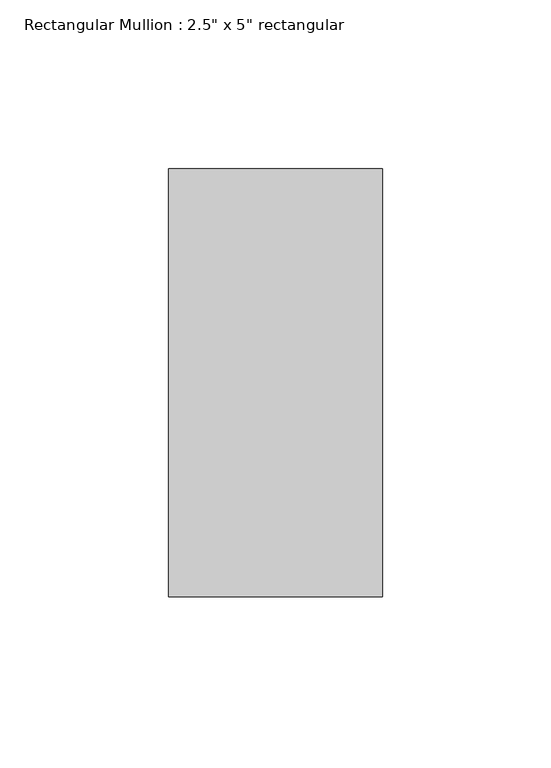
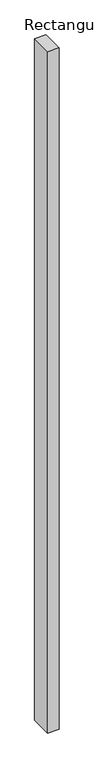
"""IFC4 building model written with IfcOpenShell, lengths in millimetres: member geometry."""

from ifc_helpers import new_model, si_unit, frame, origin, place, context, project, spatial, polyline, outline, extrude, source, transform, mapped, element, save


def member_49f7f43a(model_context):
    return source(origin(), model_context, "Body", "SweptSolid", [
        extrude(outline(polyline([(0.0, 63.5), (0.0, -63.5), (-63.5, -63.5), (-63.5, 63.5), (0.0, 63.5)])), frame((0.0, 0.0, -4035.7084783), z_axis=(0.0, 0.0, 1.0), x_axis=(1.0, 0.0, 0.0)), (0.0, 0.0, 1.0), 4035.7084783),
    ])


if __name__ == "__main__":
    model = new_model("IFC4")
    model_context = context("Model", 3, world=origin())
    ifc_project = project(units=[si_unit("LENGTHUNIT", "METRE", prefix="MILLI")], contexts=[model_context])
    site = spatial("IfcSite", under=ifc_project)
    building = spatial("IfcBuilding", under=site)
    placement = place(None, origin())
    member_shape = member_49f7f43a(model_context)
    element("IfcMember", 1, ObjectType="Rectangular Mullion : 2.5\" x 5\" rectangular", at=placement, inside=building, context=model_context, shape_type="MappedRepresentation", body=[
        mapped(member_shape, transform((0.0, 0.0, 0.0), x_axis=(1.0, 0.0, 0.0), y_axis=(0.0, 1.0, 0.0), z_axis=(0.0, 0.0, 1.0))),
    ])
    save(model, "model.ifc")

# Revit data of these elements
# Type "Rectangular Mullion : 2.5\" x 5\" rectangular"
#   built-in parameter 1007304 = 0.416667 (stored number, unit not read)
#   built-in parameter 1007301 = 0.104167 (stored number, unit not read)
#   built-in parameter 1007300 = 0.104167 (stored number, unit not read)
# Element 1 (IfcMember, "Rectangular Mullion : 2.5\" x 5\" rectangular")
#   Materials on its faces: "Iron, Ductile"
# Materials
#   "Iron, Ductile": class "Metal", colour RGB 0 0 0, transparency 0, Description = "Ductile cast iron", Cost = 0
